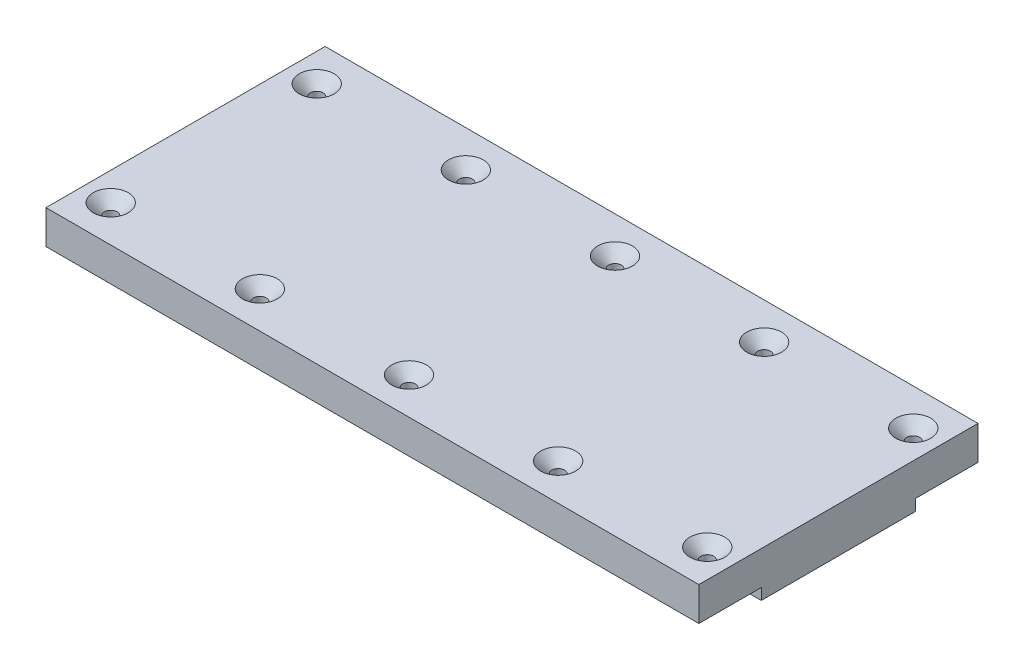
SolidWorks part; units mm, degrees
material "Plain Carbon Steel"
ref_plane "Front Plane" through (0, 0, 0) normal (0, 0, 1) x (1, 0, 0)
ref_plane "Top Plane" through (0, 0, 0) normal (0, 1, 0) x (1, 0, 0)
ref_plane "Right Plane" through (0, 0, 0) normal (1, 0, 0) x (0, 0, -1)
sketch "Plate Profile Sketch" plane through (0, 0, 0) normal (1, 0, 0) x (0, 0, -1)
  line L0 (-68.5, 0) -> (68.5, 0)
  line L1 (68.5, 0) -> (68.5, 10)
  line L2 (68.5, 10) -> (124, 10)
  line L3 (124, 10) -> (124, 40)
  line L4 (124, 40) -> (-124, 40)
  line L5 (-124, 40) -> (-124, 10)
  line L6 (-124, 10) -> (-68.5, 10)
  line L7 (-68.5, 10) -> (-68.5, 0)
  line L8 (0, 0) -> (0, 252.8487) construction
  dimension "D1" = 137
  dimension "D2" = 10
  dimension "D3" = 40
  dimension "D4" = 248
extrude "Base Plate" add sketch "Plate Profile Sketch" along normal blind 580
sketch "Mounting Holes Sketch" plane through (0, 40, 0) normal (0, 1, 0) x (1, 0, 0)
  line L0 (0, 0) -> (580, 0) construction
  line L1 (580, 124) -> (580, -124) construction
  line L2 (0, 124) -> (0, -124) construction
  circle A0 centre (25, -91.5) radius 5.7
  circle A1 centre (157.5, -91.5) radius 5.7
  circle A2 centre (422.5, -91.5) radius 5.7
  circle A3 centre (555, -91.5) radius 5.7
  circle A4 centre (290, -91.5) radius 5.7
  circle A5 centre (555, 91.5) radius 5.7
  circle A6 centre (422.5, 91.5) radius 5.7
  circle A7 centre (290, 91.5) radius 5.7
  circle A8 centre (157.5, 91.5) radius 5.7
  circle A9 centre (25, 91.5) radius 5.7
  dimension "D2" = 132.5
  dimension "D3" = 132.5
  dimension "D4" = 132.5
  dimension "D5" = 132.5
  dimension "D6" = 11.4
  dimension "D7" = 183
  dimension "D1" = 25
extrude "Mounting Holes 8xØ11" cut sketch "Mounting Holes Sketch" against normal blind 580
chamfer "Hole Chamfers 6mm" distance 9.8 angle 45 10 edges at (422.5, 40, 97.2) (25, 40, 97.2) (157.5, 40, 97.2) (290, 40, 97.2) (555, 40, 97.2) (555, 40, -97.2) (422.5, 40, -97.2) (290, 40, -97.2) (157.5, 40, -97.2) (25, 40, -97.2)
